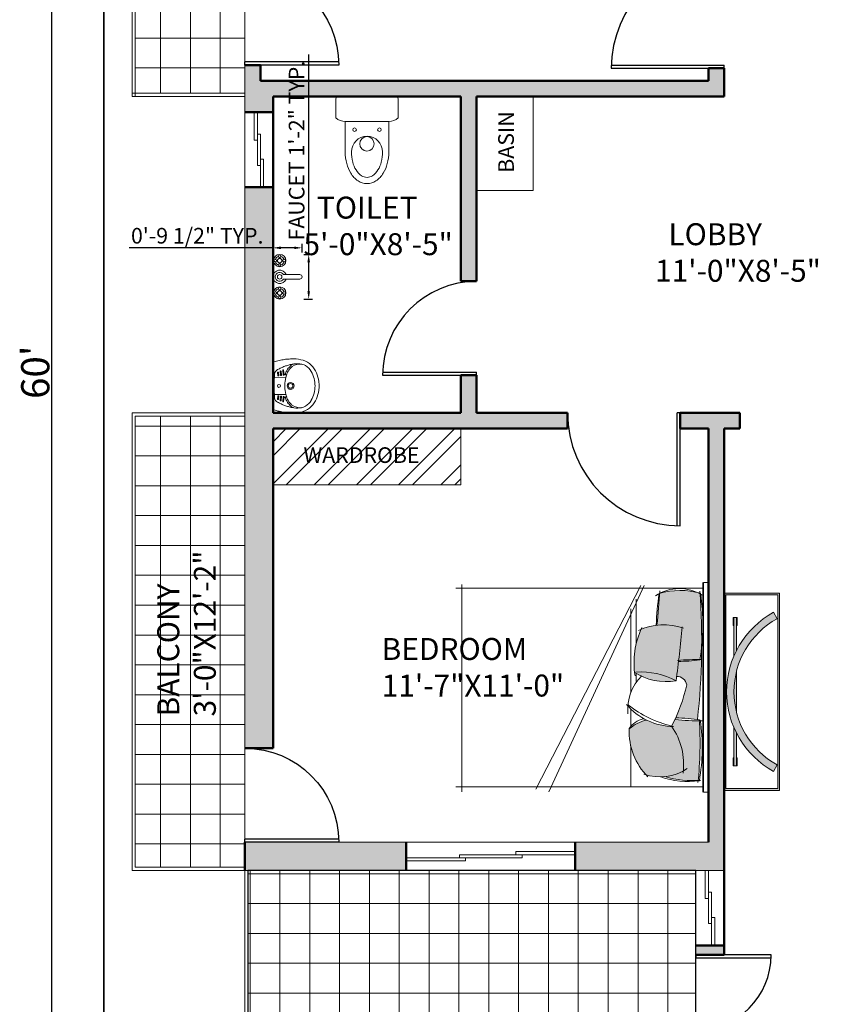
# Model space of a CAD drawing. Units: inches. Extents: x 1734 to 4011, y 1071 to 1891.
# Tile 11 of 27: x 2226 to 2484, y 1282 to 1597. Entities that reach past the tile are written whole.
import ezdxf

# ---------------------------------------------------------------- set-up
doc = ezdxf.new("R2010")
doc.units = ezdxf.units.IN
for name, color, linetype, lineweight in [('0.10', 252, 'Continuous', 9), ('0.15', 34, 'Continuous', 15), ('A-ANNO-DIMS', 2, 'Continuous', 18), ('A-AREA-IDEN', 3, 'Continuous', 18), ('A-DOOR', 3, 'Continuous', 25), ('A-FLOR-FIXT', 9, 'Continuous', 18), ('A-FLOR-OTLN', 7, 'Continuous', 25), ('A-FLOR-PATT', 252, 'Continuous', 13), ('A-FURN', 8, 'Continuous', 18), ('A-FURN-PATT', 252, 'Continuous', 13), ('A-GLAZ', 4, 'Continuous', 18), ('A-WALL', 7, 'Continuous', 50), ('A-WALL-PATT', 8, 'Continuous', 13), ('aparador', 36, 'Continuous', 9), ('C-PROP', 1, 'Continuous', 35), ('moveis', 254, 'Continuous', 5)]:
    doc.layers.add(name, color=color, linetype=linetype, lineweight=lineweight)
doc.styles.get("Standard").update_dxf_attribs({"font": 'arial.ttf'})
doc.dimstyles.new('ISO-25', dxfattribs={"dimtxt": 5, "dimasz": 2.5, "dimexe": 1.25, "dimexo": 0.625, "dimtad": 1, "dimdec": 1, "dimlunit": 3, "dimtxsty": 'Standard', "dimcen": 2.5, "dimclrt": 1, "dimadec": 0, "dimazin": 0, "dimtfac": 1, "dimtdec": 1, "dimtmove": 0, "dimatfit": 3, "dimfxl": 1, "dimarcsym": 0})
pattern_1 = [(90, (-758.361, 0), (-9.525, 0), []), (180, (-758.361, 0), (-9e-16, -9.525), [])]

# ---------------------------------------------------------------- blocks, each defined once
blk = doc.blocks.new('*D17')
at = {"layer": 'A-ANNO-DIMS', "color": 0, "lineweight": -2, "transparency": 16777216}
for p, q in [((2251.86, 1844.06), (2234.55, 1844.06)), ((2235.8, 1841.56), (2235.8, 1126.56)), ((2251.86, 1124.06), (2234.55, 1124.06))]:
    blk.add_line(p, q, dxfattribs=at)
at = {"layer": 'A-ANNO-DIMS', "color": 0, "transparency": 16777216}
for points in [[(2235.38, 1841.56), (2236.21, 1841.56), (2235.8, 1844.06)], [(2235.38, 1126.56), (2236.21, 1126.56), (2235.8, 1124.06)]]:
    blk.add_solid(points, dxfattribs=at)
at = {"layer": 'Defpoints', "color": 0, "transparency": 16777216}
for p in [(2252.48, 1844.06), (2235.8, 1124.06), (2252.48, 1124.06)]:
    blk.add_point(p, dxfattribs=at)
at = {"layer": 'A-ANNO-DIMS', "color": 0, "transparency": 16777216, "insert": (2230.58, 1484.06), "char_height": 5, "attachment_point": 5, "rotation": 90}
blk.add_mtext("{\\H1.8x;60'}", dxfattribs=at)
blk = doc.blocks.new("D1 3'")
for p, q in [((0, 36), (0, 0)), ((1, 36), (1, 0)), ((0, 0), (1, 0))]:
    blk.add_line(p, q)
blk.add_arc((0, 0), 36, 0, 90)
blk = doc.blocks.new("D2 2'6")
for p, q in [((0, 30), (0, 0)), ((1, 30), (1, 0)), ((0, 0), (1, 0))]:
    blk.add_line(p, q)
blk.add_arc((0, 0), 30, 0, 90)
blk = doc.blocks.new('camita')
at = {"layer": '0.10'}
for p, q in [((-0.85, -0.045), (0.85, -0.045)), ((-0.805, -0.045), (-0.805, -2.0485)), ((0.805, -0.045), (0.805, -2.0485)), ((-0.8271, -0.521), (0.8464, -1.2932)), ((-0.8271, -0.5476), (0.8236, -1.3992)), ((-0.7161, -0.585), (-0.3554, -0.585)), ((-0.638, -0.63), (0.0434, -0.63)), ((-0.1136, -0.585), (-0.0485, -0.585)), ((0.1749, -0.63), (0.3179, -0.63)), ((0.4739, -0.63), (0.805, -0.63)), ((-0.8354, -2), (0.8464, -2))]:
    blk.add_line(p, q, dxfattribs=at)
blk.add_lwpolyline([(-0.85, -0.0405), (0.85, -0.0405), (0.85, 0), (-0.85, 0)], close=True, dxfattribs=at)
for centre, radius, start, end in [((-0.4574, -0.2364), 0.3443, 147.50996, 213.83359), ((-0.1997, -0.2266), 0.5864, 163.92635, 197.14087), ((-0.3639, -5.8457), 5.7909, 83.80731, 94.12107), ((-0.5104, -1.7232), 1.6781, 80.12554, 98.66187), ((2.3534, -0.0532), 2.5803, 180.10628, 184.38541), ((-1.5443, -0.2452), 1.3333, 359.93941, 7.55329), ((1.5815, -0.2893), 1.3353, 170.38021, 178.99138), ((-1.4396, -0.0609), 1.7117, 352.92911, 0.39592), ((0.4524, -3.0675), 2.9996, 83.90257, 93.67595), ((0.4863, -1.6286), 1.5781, 80.16015, 98.05996), ((0.0294, -0.1377), 0.7262, 342.58415, 6.00484), ((0.1326, -0.1696), 0.6307, 339.92303, 8.74334), ((-0.0543, -0.3633), 0.4542, 159.30257, 206.50263), ((-1.3301, -9.6748), 9.4985, 82.27078, 84.93989), ((-0.007, -0.258), 0.0828, 100.01798, 179.73597), ((-0.2931, -1.4378), 1.2903, 61.97485, 77.84351), ((0.6265, -0.7518), 0.5508, 82.96906, 124.67388), ((0.3203, -0.3944), 0.4043, 341.45245, 33.45121), ((0.4585, -0.5454), 0.5842, 151.04555, 184.14969), ((-0.5341, -0.3393), 0.4875, 327.26442, 9.0473), ((-0.1986, -0.2742), 0.5159, 310.73945, 359.05759), ((-0.5673, -0.0868), 0.9057, 321.69527, 346.46261), ((-1.8672, -14.986), 14.6323, 84.65974, 85.75157), ((-0.4598, 1.4861), 1.9092, 260.95299, 268.65169), ((-0.2002, 0.064), 0.6673, 244.78094, 279.06058), ((0.179, -0.272), 0.3828, 224.52836, 275.22287), ((0.4384, -0.4834), 0.1898, 193.68485, 236.70352), ((0.5707, -0.4317), 0.3145, 192.93877, 221.96363), ((0.3612, -0.133), 0.5096, 267.25889, 315.29965)]:
    blk.add_arc(centre, radius, start, end, dxfattribs=at)
blk = doc.blocks.new("MD D 4'")
for p, q in [((0, 24), (0, 0)), ((1, 24), (1, 0)), ((47, 24), (47, 0)), ((48, 24), (48, 0)), ((0, 0), (1, 0)), ((48, 0), (47, 0))]:
    blk.add_line(p, q)
for centre, start, end in [((0, 0), 0, 90), ((48, 0), 90, 180)]:
    blk.add_arc(centre, 24, start, end)
blk = doc.blocks.new('Aparador ORGANICA Formatto')
at = {"layer": 'aparador', "ltscale": 0.3}
h = blk.add_hatch(color=256, dxfattribs=at)
h.dxf.hatch_style = 1
h.set_gradient(color1=(118, 213, 123), color2=(52, 168, 57), one_color=1, tint=0.43, name='INVCURVED')
h.paths.add_polyline_path([(0.8, 0.45), (-0.8, 0.45), (-0.8, 0), (0.8, 0)])
h.paths.add_polyline_path([(0.785, 0.435), (0.785, 0.015), (-0.785, 0.015), (-0.785, 0.435)], flags=16)
h.paths.add_polyline_path([(0.2911, 0.3699), (0.5365, 0.3699), (0.5365, 0.3757), (0.6011, 0.3757), (0.6011, 0.3699), (0.6011, 0.3499), (0.6011, 0.3441), (0.5365, 0.3441), (0.5365, 0.3499), (0.3338, 0.3499, -0.150336), (0.6449, 0.0488), (0.5923, 0.0199, 0.208852), (0.1632, 0.3499), (-0.1632, 0.3499, 0.208852), (-0.5923, 0.0199), (-0.6449, 0.0488, -0.150336), (-0.3338, 0.3499), (-0.5365, 0.3499), (-0.5365, 0.3441), (-0.6011, 0.3441), (-0.6011, 0.3499), (-0.6011, 0.3699), (-0.6011, 0.3757), (-0.5365, 0.3757), (-0.5365, 0.3699), (-0.2911, 0.3699, -0.206106)], flags=0)
h = blk.add_hatch(color=256, dxfattribs=at)
h.dxf.hatch_style = 1
h.set_gradient(color1=(135, 92, 69), color2=(0, 0, 0), one_color=1, name='INVCURVED')
h.paths.add_polyline_path([(-0.6449, 0.0488), (-0.5923, 0.0199, -0.590888), (0.5923, 0.0199), (0.6449, 0.0488, 0.590888)])
h = blk.add_hatch(color=256, dxfattribs=at)
h.dxf.hatch_style = 1
h.set_gradient(color1=(178, 189, 189), one_color=1, tint=1, name='CYLINDER')
h.paths.add_polyline_path([(-0.5365, 0.3757), (-0.6011, 0.3757), (-0.6011, 0.3699), (-0.5365, 0.3699)])
h.paths.add_polyline_path([(-0.5365, 0.3499), (-0.6011, 0.3499), (-0.6011, 0.3441), (-0.5365, 0.3441)])
h = blk.add_hatch(color=256, dxfattribs=at)
h.dxf.hatch_style = 1
h.set_gradient(color1=(118, 213, 123), color2=(31, 101, 35), one_color=1, tint=0.26, name='INVCURVED')
h.paths.add_polyline_path([(-0.2911, 0.3699), (-0.6011, 0.3699), (-0.6011, 0.3499), (-0.3338, 0.3499, -0.015999)])
h = blk.add_hatch(color=256, dxfattribs=at)
h.dxf.hatch_style = 1
h.set_gradient(color1=(118, 213, 123), color2=(31, 101, 35), one_color=1, tint=0.26, name='INVCURVED')
h.paths.add_polyline_path([(-0.1632, 0.3499), (0.1632, 0.3499, 0.122516)])
h = blk.add_hatch(color=256, dxfattribs=at)
h.dxf.hatch_style = 1
h.set_gradient(color1=(118, 213, 123), color2=(31, 101, 35), one_color=1, tint=0.26, name='INVCURVED')
h.paths.add_polyline_path([(0.6011, 0.3699), (0.2911, 0.3699, -0.015999), (0.3338, 0.3499), (0.6011, 0.3499)])
h = blk.add_hatch(color=256, dxfattribs=at)
h.dxf.hatch_style = 1
h.set_gradient(color1=(178, 189, 189), one_color=1, tint=1, name='CYLINDER')
h.paths.add_polyline_path([(0.6011, 0.3757), (0.5365, 0.3757), (0.5365, 0.3699), (0.6011, 0.3699)])
h.paths.add_polyline_path([(0.6011, 0.3499), (0.5365, 0.3499), (0.5365, 0.3441), (0.6011, 0.3441)])
for p, q in [((-0.5923, 0.0199), (-0.6449, 0.0488)), ((0.5923, 0.0199), (0.6449, 0.0488))]:
    blk.add_line(p, q, dxfattribs=at)
for points in [[(-0.6011, 0.3699), (-0.6011, 0.3757), (-0.5365, 0.3757), (-0.5365, 0.3699)], [(-0.5365, 0.3499), (-0.5365, 0.3441), (-0.6011, 0.3441), (-0.6011, 0.3499)], [(0.6011, 0.3699), (0.6011, 0.3757), (0.5365, 0.3757), (0.5365, 0.3699)], [(0.5365, 0.3499), (0.5365, 0.3441), (0.6011, 0.3441), (0.6011, 0.3499)]]:
    blk.add_lwpolyline(points, dxfattribs=at)
for radius in [0.7362, 0.6762]:
    blk.add_arc((0, -0.3063), radius, 28.84335, 151.15665, dxfattribs=at)
at = {"layer": 'moveis', "ltscale": 0.3}
for p, q in [((-0.6011, 0.3699), (-0.6011, 0.3499)), ((-0.2911, 0.3699), (-0.6011, 0.3699)), ((-0.6011, 0.3499), (-0.3338, 0.3499)), ((-0.1632, 0.3499), (0.1632, 0.3499)), ((0.2911, 0.3699), (0.6011, 0.3699)), ((0.6011, 0.3499), (0.3338, 0.3499)), ((0.6011, 0.3699), (0.6011, 0.3499))]:
    blk.add_line(p, q, dxfattribs=at)
for points in [[(-0.8, 0), (0.8, 0), (0.8, 0.45), (-0.8, 0.45)], [(-0.785, 0.015), (0.785, 0.015), (0.785, 0.435), (-0.785, 0.435)]]:
    blk.add_lwpolyline(points, close=True, dxfattribs=at)
blk = doc.blocks.new('Faucet - Bathroom top')
for p, q in [((-4.107, 0.125), (-4.375, 0.125)), ((-3.75, 0.4788), (-3.75, 0.75)), ((-3.5, 0.482), (-3.5, 0.75)), ((-3.1461, 0.125), (-2.875, 0.125)), ((3.143, 0.125), (2.875, 0.125)), ((3.5, 0.4788), (3.5, 0.75)), ((3.75, 0.482), (3.75, 0.75)), ((4.1039, 0.125), (4.375, 0.125)), ((-4.1039, -0.125), (-4.375, -0.125)), ((-3.75, -0.4821), (-3.75, -0.75)), ((-3.5, -0.4789), (-3.5, -0.75)), ((-3.143, -0.125), (-2.875, -0.125)), ((-0.5, -0.8639), (-0.5, -4.5)), ((0.5, -4.5), (0.5, -0.8631)), ((3.1461, -0.125), (2.875, -0.125)), ((3.5, -0.4821), (3.5, -0.75)), ((3.75, -0.4789), (3.75, -0.75)), ((4.107, -0.125), (4.375, -0.125))]:
    blk.add_line(p, q)
for centre, radius in [((-3.625, 0), 1.375), ((-4.625, 0), 0.2795), ((-3.625, 0), 0.5), ((-3.625, 1), 0.2795), ((-2.625, 0), 0.2795), ((0, 0), 0.5), ((3.625, 0), 1.375), ((2.625, 0), 0.2795), ((3.625, 0), 0.5), ((3.625, 1), 0.2795), ((4.625, 0), 0.2795), ((-3.625, -1), 0.2795), ((3.625, -1), 0.2795)]:
    blk.add_circle(centre, radius)
for centre, radius, start, end in [((-3.625, 0), 1, 105.2407, 164.2093), ((-3.625, 0), 1, 16.44125, 74.07887), ((0, 0), 1.5, 289.6514, 250.3603), ((0, 0), 1, 300.3431, 239.7554), ((3.625, 0), 1, 106.12, 164.0884), ((3.625, 0), 1, 16.23422, 73.90469), ((-3.625, 0), 1, 196.2342, 253.9047), ((-3.625, 0), 1, 286.12, 344.0884), ((3.625, 0), 1, 196.4413, 254.0789), ((3.625, 0), 1, 285.2407, 344.2093), ((0, -4.5), 0.5, 180, 0)]:
    blk.add_arc(centre, radius, start, end)
blk = doc.blocks.new('lavamanos 2')
at = {"layer": '0.15'}
for p, q in [((0, 0.2335), (0, -0.2335)), ((-0.1304, 0.11), (-0.1315, 0.11)), ((-0.1127, 0.112), (-0.1067, 0.1581)), ((-0.1037, 0.1109), (-0.0978, 0.157)), ((-0.0857, 0.1085), (-0.0807, 0.1466)), ((-0.0767, 0.1074), (-0.0718, 0.1455)), ((-0.0587, 0.105), (-0.0548, 0.1351)), ((-0.0497, 0.1039), (-0.0458, 0.134)), ((-0.0142, 0.087), (-0.13, 0.086)), ((-0.0142, -0.087), (-0.13, -0.086)), ((-0.1304, -0.11), (-0.1315, -0.11)), ((-0.1127, -0.112), (-0.1067, -0.1581)), ((-0.1037, -0.1109), (-0.0978, -0.157)), ((-0.0857, -0.1085), (-0.0807, -0.1466)), ((-0.0767, -0.1074), (-0.0718, -0.1455)), ((-0.0587, -0.105), (-0.0548, -0.1351)), ((-0.0497, -0.1039), (-0.0458, -0.134))]:
    blk.add_line(p, q, dxfattribs=at)
for centre, radius in [((-0.178, 0), 0.035), ((-0.178, 0), 0.0235), ((-0.06, 0), 0.015)]:
    blk.add_circle(centre, radius, dxfattribs=at)
for centre, radius, start, end in [((-0.1663, 0.0005), 0.3024, 136.57187, 154.32772), ((-0.2419, 0.0663), 0.2023, 108.1945, 135.36859), ((-0.2422, 0.0655), 0.1638, 121.99295, 150.58892), ((-0.2657, 0.1037), 0.119, 92.47742, 122.14108), ((-0.2035, -0.0862), 0.3593, 91.20299, 106.42552), ((-0.2765, 0.0677), 0.1528, 57.2491, 95.54005), ((-0.2442, -0.0128), 0.2368, 77.24819, 96.46321), ((-0.2208, -0.6855), 0.9585, 86.55138, 89.41308), ((-0.2765, 0.0677), 0.1678, 56.87663, 64.99714), ((-0.2222, 0.0026), 0.2177, 71.98488, 82.01242), ((-0.3662, -0.002), 0.2777, 40.35252, 49.22548), ((-0.2121, -0.5476), 0.8204, 83.12241, 86.5796), ((-0.3103, -0.315), 0.5472, 69.51913, 73.49118), ((5.8279, 30.215), 30.5319, 258.77821, 258.87599), ((-0.1265, -0.0657), 0.3287, 69.06009, 78.82181), ((-0.0202, 0.212), 0.0314, 54.79491, 69.06009), ((-0.005, 0.2335), 0.005, 0, 54.79491), ((-0.0557, -0.0178), 0.4111, 158.70106, 171.31016), ((-0.1999, 0.0263), 0.2202, 147.11565, 167.44248), ((-0.3662, -0.002), 0.2627, 40.35252, 49.00458), ((-0.2374, 0.11), 0.0921, 27.31862, 39.11562), ((-0.3494, 0.0363), 0.2258, 22.33605, 30.8927), ((-0.2374, 0.11), 0.1071, 27.57433, 39.11562), ((-0.3494, 0.0363), 0.2408, 22.19214, 30.78376), ((-1.2664, -0.2389), 1.1824, 16.36313, 17.77674), ((-0.1315, 0.117), 0.007, 197.40991, 270.49494), ((-0.1305, 0.117), 0.007, 270.49494, 17.39527), ((-1.2664, -0.2389), 1.1974, 17.39527, 17.80495), ((-0.2991, -0.2855), 0.5156, 65.23004, 69.53785), ((-0.1082, 0.1115), 0.0045, 172.61396, 352.61396), ((-0.1022, 0.1575), 0.0045, 352.61396, 172.61396), ((-0.0812, 0.108), 0.0045, 172.61396, 352.61396), ((-0.2784, -0.2408), 0.4663, 60.24131, 65.2382), ((-0.0763, 0.146), 0.0045, 352.61396, 172.61396), ((-0.0542, 0.1045), 0.0045, 172.61396, 352.61396), ((-0.0503, 0.1345), 0.0045, 352.61396, 172.61396), ((-0.0648, 0.1184), 0.049, 1.58272, 68.62081), ((-2.1477, 0.0009), 2.1352, 359.97535, 3.19009), ((-0.2093, 0.0056), 0.2558, 171.31016, 181.26266), ((-0.2093, -0.0056), 0.2558, 178.73734, 188.68984), ((0.4664, -0.0834), 0.8953, 169.86317, 174.65802), ((0.4664, 0.0834), 0.8953, 185.34198, 190.13683), ((0.1853, 0.1648), 0.325, 192.53887, 196.70718), ((0.3887, 0.121), 0.517, 185.50529, 189.81306), ((-0.7181, -0.0071), 0.5987, 0.67647, 3.82165), ((-0.7181, 0.0071), 0.5987, 356.17835, 359.32353), ((-2.1477, -0.0009), 2.1352, 356.80991, 0.02465), ((-0.0557, 0.0178), 0.4111, 188.68984, 201.29894), ((-0.1999, -0.0263), 0.2202, 192.55752, 212.88435), ((-1.2664, 0.2389), 1.1824, 342.22326, 343.63687), ((0.1853, -0.1648), 0.325, 163.29282, 167.46113), ((0.3887, -0.1209), 0.517, 170.18694, 174.49471), ((-0.1663, -0.0005), 0.3024, 205.67228, 223.42813), ((-0.2422, -0.0655), 0.1638, 209.41108, 238.00705), ((-0.2765, -0.0677), 0.1528, 264.45995, 302.7509), ((-0.3662, 0.002), 0.2627, 310.99542, 319.64748), ((-0.3662, 0.002), 0.2777, 310.77452, 319.64748), ((-0.2374, -0.1099), 0.0921, 320.88438, 332.68138), ((-0.3494, -0.0363), 0.2258, 329.1073, 337.66395), ((-0.3103, 0.315), 0.5472, 286.50882, 290.48087), ((-0.2374, -0.1099), 0.1071, 320.88438, 332.42567), ((-0.3494, -0.0363), 0.2408, 329.21624, 337.80786), ((-0.1315, -0.117), 0.007, 89.50506, 162.59009), ((-0.1305, -0.117), 0.007, 342.60473, 89.50506), ((-1.2664, 0.2389), 1.1974, 342.19505, 342.60473), ((-0.2991, 0.2855), 0.5156, 290.46215, 294.76996), ((-0.1082, -0.1115), 0.0045, 7.38604, 187.38604), ((-0.1022, -0.1575), 0.0045, 187.38604, 7.38604), ((-0.0812, -0.108), 0.0045, 7.38604, 187.38604), ((-0.2784, 0.2408), 0.4663, 294.7618, 299.75869), ((-0.0763, -0.146), 0.0045, 187.38604, 7.38604), ((-0.0542, -0.1045), 0.0045, 7.38604, 187.38604), ((-0.0503, -0.1345), 0.0045, 187.38604, 7.38604), ((-0.0648, -0.1184), 0.049, 291.37919, 358.41728), ((-0.2419, -0.0663), 0.2023, 224.63141, 251.8055), ((-0.2657, -0.1036), 0.119, 237.85892, 267.52258), ((-0.2035, 0.0862), 0.3593, 253.57448, 268.79701), ((-0.2442, 0.0128), 0.2368, 263.53679, 282.75181), ((-0.2208, 0.6855), 0.9585, 270.58692, 273.44862), ((-0.2765, -0.0677), 0.1678, 295.00286, 303.12337), ((-0.2222, -0.0026), 0.2177, 277.98758, 288.01512), ((-0.2121, 0.5476), 0.8204, 273.4204, 276.87759), ((5.8279, -30.215), 30.5319, 101.12401, 101.22179), ((-0.1265, 0.0657), 0.3287, 281.17819, 290.93991), ((-0.0202, -0.212), 0.0314, 290.93991, 305.20509), ((-0.005, -0.2335), 0.005, 305.20509, 0)]:
    blk.add_arc(centre, radius, start, end, dxfattribs=at)
blk = doc.blocks.new('rreerr')
blk.add_lwpolyline([(2512.8529, 833.5601, 0.205217), (2512.9279, 833.5883), (2512.9279, 833.7401, 0.414214), (2512.9079, 833.7601), (2512.4479, 833.7601, 0.414214), (2512.4279, 833.7401), (2512.4279, 833.5883, 0.205217), (2512.5029, 833.5601)], format="xyb")
for points in [[(2512.5468, 833.1438, 0.107027), (2512.6056, 833.0819, 0.150548), (2512.6779, 833.0596, 0.150548), (2512.7502, 833.0819, 0.107027), (2512.809, 833.1438, 0.075071), (2512.8412, 833.2206, 0.0618), (2512.8529, 833.3151), (2512.8529, 833.5601), (2512.5029, 833.5601), (2512.5029, 833.3151, 0.0618), (2512.5146, 833.2206, 0.075071)], [(2512.5631, 833.2328, 0.075071), (2512.5895, 833.1698, 0.107027), (2512.6338, 833.1232, 0.150548), (2512.6779, 833.1096, 0.150548), (2512.722, 833.1232, 0.107027), (2512.7663, 833.1698, 0.075071), (2512.7927, 833.2328, 0.0618), (2512.8029, 833.3151, 1), (2512.5529, 833.3151, 0.0618)]]:
    blk.add_lwpolyline(points, format="xyb", close=True)
for centre, radius in [((2512.5779, 833.493), 0.0146), ((2512.7779, 833.493), 0.0146), ((2512.6775, 833.3793), 0.0579)]:
    blk.add_circle(centre, radius)
blk = doc.blocks.new('*D89')
at = {"layer": 'A-ANNO-DIMS', "color": 0, "lineweight": -2, "transparency": 16777216}
for p, q in [((2317.87, 1521.62), (2317.87, 1585.44)), ((2316.36, 1521.62), (2319.12, 1521.62)), ((2317.87, 1509.88), (2317.87, 1519.12)), ((2316.36, 1507.38), (2319.12, 1507.38))]:
    blk.add_line(p, q, dxfattribs=at)
at = {"layer": 'A-ANNO-DIMS', "color": 0, "transparency": 16777216}
for points in [[(2317.46, 1519.12), (2318.29, 1519.12), (2317.87, 1521.62)], [(2317.46, 1509.88), (2318.29, 1509.88), (2317.87, 1507.38)]]:
    blk.add_solid(points, dxfattribs=at)
at = {"layer": 'Defpoints', "color": 0, "transparency": 16777216}
for p in [(2315.74, 1521.62), (2317.87, 1521.62), (2315.74, 1507.38)]:
    blk.add_point(p, dxfattribs=at)
at = {"layer": 'A-ANNO-DIMS', "color": 1, "transparency": 16777216, "insert": (2314.66, 1554.78), "char_height": 5, "attachment_point": 5, "rotation": 90}
blk.add_mtext('FAUCET 1\'-2" TYP.', dxfattribs=at)
blk = doc.blocks.new('*D90')
at = {"layer": 'A-ANNO-DIMS', "color": 0, "lineweight": -2, "transparency": 16777216}
for p, q in [((2306.48, 1522.24), (2306.48, 1525)), ((2315.74, 1522.24), (2315.74, 1525)), ((2306.48, 1523.75), (2260.6, 1523.75)), ((2313.24, 1523.75), (2308.98, 1523.75))]:
    blk.add_line(p, q, dxfattribs=at)
at = {"layer": 'A-ANNO-DIMS', "color": 0, "transparency": 16777216}
for points in [[(2308.98, 1524.17), (2308.98, 1523.34), (2306.48, 1523.75)], [(2313.24, 1524.17), (2313.24, 1523.34), (2315.74, 1523.75)]]:
    blk.add_solid(points, dxfattribs=at)
at = {"layer": 'Defpoints', "color": 0, "transparency": 16777216}
for p in [(2306.48, 1523.75), (2306.48, 1521.62), (2315.74, 1521.62)]:
    blk.add_point(p, dxfattribs=at)
at = {"layer": 'A-ANNO-DIMS', "color": 1, "transparency": 16777216, "insert": (2282.29, 1526.96), "char_height": 5, "attachment_point": 5}
blk.add_mtext('0\'-9 1/2" TYP.', dxfattribs=at)

msp = doc.modelspace()

# ---------------------------------------------------------------- hatches: boundary and pattern name
at = {"layer": 'A-FLOR-PATT'}
h = msp.add_hatch(dxfattribs=at)
h.set_pattern_fill('ANSI37', color=256, scale=3, angle=45)
h.set_pattern_definition(pattern_1)
h.paths.add_polyline_path([(2297.48, 1758.06), (2262.48, 1758.06), (2262.48, 1573.06), (2297.48, 1573.06), (2297.48, 1582.06), (2297.48, 1583.06)])
h.paths.add_polyline_path([(2292.19, 1643.04), (2292.19, 1697.75), (2266.07, 1697.75), (2266.07, 1643.04)], flags=24)
h = msp.add_hatch(dxfattribs=at)
h.set_pattern_fill('ANSI37', color=256, scale=3, angle=45)
h.set_pattern_definition(pattern_1)
h.paths.add_polyline_path([(2262.48, 1326.06), (2297.48, 1326.06), (2297.48, 1470.06), (2262.48, 1470.06)])
h.paths.add_polyline_path([(2292.19, 1371.73), (2292.19, 1426.44), (2266.07, 1426.44), (2266.07, 1371.73)], flags=24)
h = msp.add_hatch(dxfattribs=at)
h.set_pattern_fill('ANSI37', color=256, scale=3, angle=45)
h.set_pattern_definition(pattern_1)
h.paths.add_polyline_path([(2262.48, 1326.06), (2297.48, 1326.06), (2297.48, 1470.06), (2262.48, 1470.06)])
h.paths.add_polyline_path([(2292.19, 1371.73), (2292.19, 1426.44), (2266.07, 1426.44), (2266.07, 1371.73)], flags=24)
h = msp.add_hatch(dxfattribs=at)
h.set_pattern_fill('ANSI37', color=256, scale=3, angle=45)
h.set_pattern_definition(pattern_1)
h.paths.add_polyline_path([(2441.48, 1241.06), (2441.48, 1325.06), (2298.48, 1325.06), (2298.48, 1125.06), (2428.48, 1125.06), (2428.48, 1133.06), (2484.48, 1133.06), (2484.48, 1202.06), (2494.48, 1202.06), (2494.48, 1241.06)])
h.paths.add_polyline_path([(2467.59, 1146.53), (2480.18, 1146.53), (2480.18, 1156.83), (2467.59, 1156.83)], flags=24)
h.paths.add_polyline_path([(2467.58, 1215.53), (2479.78, 1215.53), (2479.78, 1225.83), (2467.58, 1225.83)], flags=24)
h.paths.add_polyline_path([(2330.54, 1224.14), (2390.38, 1224.14), (2390.38, 1250.26), (2330.54, 1250.26)], flags=24)
at = {"layer": 'A-FURN-PATT'}
h = msp.add_hatch(dxfattribs=at)
h.set_pattern_fill('ANSI32', color=256)
h.set_pattern_definition([(45, (-758.361, 0), (-6.735192, 6.735192), []), (45, (-753.871, 0), (-6.735192, 6.735192), [])])
h.paths.add_polyline_path([(2366.48, 1466.06), (2306.48, 1466.06), (2306.48, 1448.06), (2366.48, 1448.06)])
h.paths.add_polyline_path([(2310.37, 1452.28), (2359.82, 1452.28), (2359.82, 1462.58), (2310.37, 1462.58)], flags=24)
h.paths.add_polyline_path([(2525.12, 1646.17), (2525.12, 1700.88), (2499, 1700.88), (2499, 1646.17)], flags=9)
h.paths.add_polyline_path([(2555.1, 1646.17), (2555.1, 1700.88), (2528.98, 1700.88), (2528.98, 1646.17)], flags=9)
h.paths.add_polyline_path([(2492.08, 1807.82), (2546.48, 1807.82), (2546.48, 1833.94), (2492.08, 1833.94)], flags=9)
h.paths.add_polyline_path([(2464.41, 1783), (2507.08, 1783), (2507.08, 1791.24), (2464.41, 1791.24)], flags=9)
h.paths.add_polyline_path([(2467.59, 1146.53), (2480.18, 1146.53), (2480.18, 1156.83), (2467.59, 1156.83)], flags=9)
h.paths.add_polyline_path([(2467.58, 1215.53), (2479.78, 1215.53), (2479.78, 1225.83), (2467.58, 1225.83)], flags=9)
h.paths.add_polyline_path([(2292.19, 1646.17), (2292.19, 1700.88), (2266.07, 1700.88), (2266.07, 1646.17)], flags=9)
h.paths.add_polyline_path([(2504.62, 1567.64), (2559.02, 1567.64), (2559.02, 1593.76), (2504.62, 1593.76)], flags=9)
h.paths.add_polyline_path([(2562.71, 1614.15), (2583.08, 1614.15), (2583.08, 1624.45), (2562.71, 1624.45)], flags=9)
h.paths.add_polyline_path([(2522.41, 1650.28), (2571.86, 1650.28), (2571.86, 1660.58), (2522.41, 1660.58)], flags=9)
h.paths.add_polyline_path([(2504.36, 1707.67), (2564.2, 1707.67), (2564.2, 1733.79), (2504.36, 1733.79)], flags=9)
h.paths.add_polyline_path([(2381.34, 1790.51), (2430.31, 1790.51), (2430.31, 1816.63), (2381.34, 1816.63)], flags=9)
h.paths.add_polyline_path([(2291.99, 1790.51), (2340.95, 1790.51), (2340.95, 1816.63), (2291.99, 1816.63)], flags=9)
h.paths.add_polyline_path([(2330.54, 1224.14), (2390.38, 1224.14), (2390.38, 1250.26), (2330.54, 1250.26)], flags=9)
h.paths.add_polyline_path([(2425.61, 1508.95), (2480.02, 1508.95), (2480.02, 1535.07), (2425.61, 1535.07)], flags=9)
h.paths.add_polyline_path([(2505.48, 1357.1), (2574.53, 1357.1), (2574.53, 1383.22), (2505.48, 1383.22)], flags=9)
h.paths.add_polyline_path([(2530.46, 1484.55), (2584.86, 1484.55), (2584.86, 1510.67), (2530.46, 1510.67)], flags=9)
h.paths.add_polyline_path([(2349.79, 1659.95), (2415.08, 1659.95), (2415.08, 1686.07), (2349.79, 1686.07)], flags=9)
h = msp.add_hatch(color=256, dxfattribs=at)
h.dxf.hatch_style = 1
h.paths.add_polyline_path([(2442.8, 1413.3, 0.020657), (2441.8, 1413.8, 0.131047), (2429.91, 1413.42, -0.004387), (2429.05, 1403.35, -0.113891), (2437.05, 1402.48, -0.006967), (2435.98, 1392.12, -0.016701), (2442.76, 1392.39, 0.015442), (2443.32, 1396.43, 0.01851)])
h.paths.add_polyline_path([(2437.05, 1402.48, 0.189536), (2423.97, 1401.96, 0.134508), (2421.91, 1388.23, 0.181694), (2435.14, 1385.53, 0.011408)])
h.paths.add_polyline_path([(2433.81, 1370.98, -0.104045), (2425.71, 1373.05, 0.127326), (2420.2, 1370.19, 0.202559), (2425.58, 1355.53, 0.194952), (2437.48, 1356.81, 0.173835)])
h.paths.add_polyline_path([(2442.59, 1372.74, -0.029051), (2434.79, 1373.25, -0.011742), (2433.71, 1371.12, -0.175864), (2437.48, 1356.81, -0.098488), (2431.53, 1355, 0.094792), (2442.21, 1353.78, 0.040212)])
h = msp.add_hatch(color=256, dxfattribs=at)
h.dxf.hatch_style = 1
h.paths.add_polyline_path([(2435.02, 1373.75, -0.033321), (2441.99, 1373.16, 0.021136), (2443.26, 1392.39, 0.017944), (2435.98, 1392.12, -0.003455), (2435.34, 1386.99, -0.362577), (2438.53, 1384.29, -0.054862)])
at = {"layer": 'A-WALL-PATT'}
h = msp.add_hatch(color=256, dxfattribs=at)
h.dxf.hatch_style = 1
h.paths.add_polyline_path([(2306.48, 1543.06), (2297.48, 1543.06), (2297.48, 1364.06), (2306.48, 1364.06), (2306.48, 1466.06), (2400.48, 1466.06), (2400.48, 1471.06), (2371.48, 1471.06), (2371.48, 1483.06), (2366.48, 1483.06), (2366.48, 1471.06), (2306.48, 1471.06)])
h.paths.add_polyline_path([(2348.98, 1334.06), (2297.48, 1334.06), (2297.48, 1325.06), (2348.98, 1325.06)])
h.paths.add_polyline_path([(2450.48, 1466.06), (2455.48, 1466.06), (2455.48, 1471.06), (2436.48, 1471.06), (2436.48, 1466.06), (2445.48, 1466.06), (2445.48, 1334.06), (2402.98, 1334.06), (2402.98, 1325.06), (2450.48, 1325.06)])
h.paths.add_polyline_path([(2450.48, 1301.06), (2441.48, 1301.06), (2441.48, 1298.06), (2450.48, 1298.06)])
h.paths.add_polyline_path([(2450.48, 1581.06), (2445.48, 1581.06), (2445.48, 1577.06), (2302.48, 1577.06), (2302.48, 1582.06), (2297.48, 1582.06), (2297.48, 1567.06), (2306.48, 1567.06), (2306.48, 1572.06), (2366.48, 1572.06), (2366.48, 1513.06), (2371.48, 1513.06), (2371.48, 1572.06), (2450.48, 1572.06)])
h.paths.add_polyline_path([(2302.48, 1636.07), (2297.48, 1636.07), (2297.48, 1612.06), (2302.48, 1612.06)])
h.paths.add_polyline_path([(2363.48, 1763.06), (2294.05, 1763.06), (2294.05, 1758.06), (2297.48, 1758.06), (2297.48, 1684.07), (2302.48, 1684.07), (2302.48, 1758.06), (2363.48, 1758.06)])
h.paths.add_polyline_path([(2461.48, 1250.06), (2441.48, 1250.06), (2441.48, 1241.06), (2461.48, 1241.06)])

# ---------------------------------------------------------------- linework, layer by layer
at = {"layer": 'A-FLOR-OTLN'}
msp.add_lwpolyline([(2441.48, 1241.06), (2441.48, 1325.06), (2298.48, 1325.06), (2298.48, 1125.06), (2441.48, 1125.06)], dxfattribs=at)
at = {"layer": 'A-FURN'}
for p, q in [((2261.48, 1572.06), (2261.48, 1844.06)), ((2262.48, 1572.06), (2262.48, 1758.06)), ((2297.48, 1582.06), (2297.48, 1758.06)), ((2297.48, 1124.06), (2297.48, 1582.06)), ((2261.48, 1573.06), (2297.48, 1573.06)), ((2261.48, 1471.06), (2297.48, 1471.06)), ((2261.48, 1325.06), (2261.48, 1471.06)), ((2262.48, 1326.06), (2262.48, 1470.06)), ((2262.48, 1470.06), (2297.48, 1470.06)), ((2306.48, 1448.06), (2366.48, 1448.06)), ((2297.48, 1334.06), (2445.48, 1334.06)), ((2261.48, 1325.06), (2450.48, 1325.06)), ((2262.48, 1326.06), (2297.48, 1326.06)), ((2298.48, 1125.06), (2298.48, 1325.06)), ((2441.48, 1325.06), (2441.48, 1298.06))]:
    msp.add_line(p, q, dxfattribs=at)
at = {"layer": 'A-GLAZ'}
for p, q in [((2261.48, 1572.06), (2297.48, 1572.06)), ((2389.48, 1542.06), (2389.48, 1572.06)), ((2300.48, 1558.06), (2300.48, 1567.06)), ((2301.48, 1550.06), (2301.48, 1567.06)), ((2302.48, 1560.06), (2301.48, 1560.06)), ((2302.48, 1543.06), (2302.48, 1560.06)), ((2301.48, 1558.06), (2300.48, 1558.06)), ((2302.48, 1550.06), (2301.48, 1550.06)), ((2303.48, 1552.06), (2302.48, 1552.06)), ((2303.48, 1543.06), (2303.48, 1552.06)), ((2371.48, 1542.06), (2389.48, 1542.06)), ((2366.48, 1448.06), (2366.48, 1466.06)), ((2365.98, 1330.06), (2365.98, 1329.06)), ((2365.98, 1330.06), (2402.98, 1330.06)), ((2383.98, 1331.06), (2383.98, 1330.06)), ((2383.98, 1331.06), (2402.98, 1331.06)), ((2385.98, 1330.06), (2385.98, 1329.06)), ((2348.98, 1329.06), (2385.98, 1329.06)), ((2348.98, 1328.06), (2367.98, 1328.06)), ((2367.98, 1329.06), (2367.98, 1328.06)), ((2444.48, 1316.06), (2444.48, 1325.06)), ((2445.48, 1308.06), (2445.48, 1325.06)), ((2446.48, 1318.06), (2445.48, 1318.06)), ((2446.48, 1301.06), (2446.48, 1318.06)), ((2445.48, 1316.06), (2444.48, 1316.06)), ((2446.48, 1308.06), (2445.48, 1308.06)), ((2447.48, 1310.06), (2446.48, 1310.06)), ((2447.48, 1301.06), (2447.48, 1310.06))]:
    msp.add_line(p, q, dxfattribs=at)
at = {"layer": 'A-WALL'}
for p, q in [((2297.48, 1582.06), (2302.48, 1582.06)), ((2302.48, 1577.06), (2302.48, 1582.06)), ((2445.48, 1581.06), (2450.48, 1581.06)), ((2445.48, 1577.06), (2445.48, 1581.06)), ((2450.48, 1572.06), (2450.48, 1581.06)), ((2302.48, 1577.06), (2445.48, 1577.06)), ((2306.48, 1471.06), (2306.48, 1572.06)), ((2306.48, 1572.06), (2366.48, 1572.06)), ((2366.48, 1513.06), (2366.48, 1572.06)), ((2371.48, 1513.06), (2371.48, 1572.06)), ((2371.48, 1572.06), (2450.48, 1572.06)), ((2306.48, 1567.06), (2297.48, 1567.06)), ((2306.48, 1543.06), (2297.48, 1543.06)), ((2366.48, 1513.06), (2371.48, 1513.06)), ((2366.48, 1483.06), (2371.48, 1483.06)), ((2366.48, 1471.06), (2366.48, 1483.06)), ((2371.48, 1471.06), (2371.48, 1483.06)), ((2306.48, 1471.06), (2366.48, 1471.06)), ((2371.48, 1471.06), (2400.48, 1471.06)), ((2400.48, 1466.06), (2400.48, 1471.06)), ((2436.48, 1471.06), (2455.48, 1471.06)), ((2436.48, 1466.06), (2436.48, 1471.06)), ((2455.48, 1466.06), (2455.48, 1471.06)), ((2306.48, 1466.06), (2400.48, 1466.06)), ((2306.48, 1364.06), (2306.48, 1466.06)), ((2436.48, 1466.06), (2445.48, 1466.06)), ((2445.48, 1334.06), (2445.48, 1466.06)), ((2450.48, 1466.06), (2455.48, 1466.06)), ((2450.48, 1298.06), (2450.48, 1466.06)), ((2297.48, 1364.06), (2306.48, 1364.06)), ((2297.48, 1325.06), (2297.48, 1334.06)), ((2348.98, 1334.06), (2348.98, 1325.06)), ((2402.98, 1334.06), (2402.98, 1325.06)), ((2450.48, 1301.06), (2441.48, 1301.06)), ((2450.48, 1298.06), (2441.48, 1298.06))]:
    msp.add_line(p, q, dxfattribs=at)
at = {"layer": 'C-PROP'}
msp.add_lwpolyline([(2428.48, 1124.06), (2252.48, 1124.06), (2252.48, 1844.06), (2612.48, 1844.06), (2612.48, 1124.06), (2428.48, 1124.06)], dxfattribs=at)

# ---------------------------------------------------------------- block references
at = {"layer": 'A-DOOR'}
for name, p, rotation in [("D1 3'", (2450.48, 1581.06), 90), ("D2 2'6", (2371.48, 1483.06), 90.00000000000003), ("D1 3'", (2436.48, 1471.06), 180), ("MD D 4'", (2441.48, 1298.06), 270)]:
    msp.add_blockref(name, p, dxfattribs=dict(at, rotation=rotation))
at = {"layer": 'A-DOOR', "xscale": -1, "rotation": 270}
for p in [(2297.48, 1582.06), (2297.48, 1334.06)]:
    msp.add_blockref("D2 2'6", p, dxfattribs=at)
at = {"layer": 'A-FLOR-FIXT', "xscale": 39.701, "yscale": 39.701, "zscale": 39.701}
msp.add_blockref('rreerr', (-97419.34, -31529.05), dxfattribs=at)
at = {"layer": 'A-FLOR-FIXT'}
for name, p, xscale, yscale, zscale, rotation in [('Faucet - Bathroom top', (2308.62, 1514.5), 1.424049708253414, 1.424049708253414, 1.424049708253414, 90), ('lavamanos 2', (2306.48, 1479.69), 31.61240364394164, 31.61240364394164, 31.61240364394164, 179.99990349049)]:
    msp.add_blockref(name, p, dxfattribs=dict(at, xscale=xscale, yscale=yscale, zscale=zscale, rotation=rotation))
at = {"layer": 'A-FURN'}
for name, p, xscale, yscale, zscale, rotation in [('camita', (2445.48, 1383.45), 39.375, 39.375, 39.375, 270), ('Aparador ORGANICA Formatto', (2468.2, 1382.06), 39.3701, 39.3701, 39.3701, 90)]:
    msp.add_blockref(name, p, dxfattribs=dict(at, xscale=xscale, yscale=yscale, zscale=zscale, rotation=rotation))

# ---------------------------------------------------------------- texts
at = {"layer": 'A-AREA-IDEN', "attachment_point": 1, "rotation": 90}
for s, insert, char_height in [('BASIN', (2378.37, 1547.7), 5), ('BALCONY\\P3\'-0"X12\'-2"', (2269.55, 1374.19), 7)]:
    msp.add_mtext_dynamic_manual_height_columns(s, width=86.9528, gutter_width=12.5, heights=[0], dxfattribs=dict(at, insert=insert, char_height=char_height))
at = {"layer": 'A-AREA-IDEN', "attachment_point": 1}
for s, insert, char_height in [('  TOILET\\P5\'-0"X8\'-5"', (2316.21, 1540.08), 7), ('  LOBBY\\P11\'-0"X8\'-5"', (2428.42, 1531.59), 7), ('   WARDROBE', (2311.62, 1460.1), 5), ('BEDROOM\\P11\'-7"X11\'-0"', (2341.16, 1399.22), 7)]:
    msp.add_mtext_dynamic_manual_height_columns(s, width=86.9528, gutter_width=12.5, heights=[0], dxfattribs=dict(at, insert=insert, char_height=char_height))

# ---------------------------------------------------------------- dimensions: what is measured, and where the dimension line sits
at = {"layer": 'A-ANNO-DIMS'}
for base, p1, p2, angle, text, override, picture, middle in [((2235.8, 1124.06), (2252.48, 1844.06), (2252.48, 1124.06), 90, '{\\H1.8x;<>}', {"dimclrd": 0, "dimclre": 0, "dimclrt": 0}, '*D17', (2230.58, 1484.06)), ((2317.87, 1521.62), (2315.74, 1507.38), (2315.74, 1521.62), 90, 'FAUCET <> TYP.', {"dimdec": 1, "dimrnd": 0, "dimzin": 1, "dimlunit": 4, "dimfrac": 2}, '*D89', (2314.66, 1554.78)), ((2306.48, 1523.75), (2315.74, 1521.62), (2306.48, 1521.62), 180, '<> TYP.', {"dimdec": 1, "dimrnd": 0, "dimzin": 1, "dimlunit": 4, "dimfrac": 2}, '*D90', (2282.29, 1526.96))]:
    dim = msp.add_linear_dim(base=base, p1=p1, p2=p2, angle=angle, text=text, dimstyle='ISO-25', override=override, dxfattribs=at)
    dim.commit()
    dim.dimension.update_dxf_attribs({"geometry": picture, "text_midpoint": middle})

doc.saveas('drawing.dxf')
